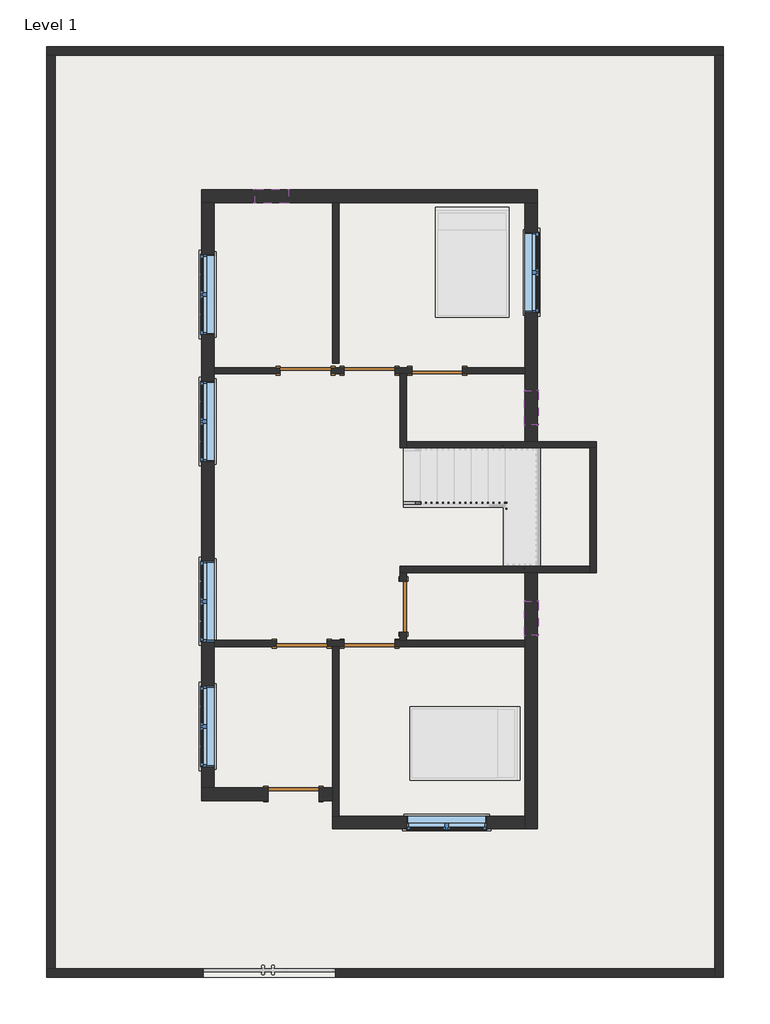
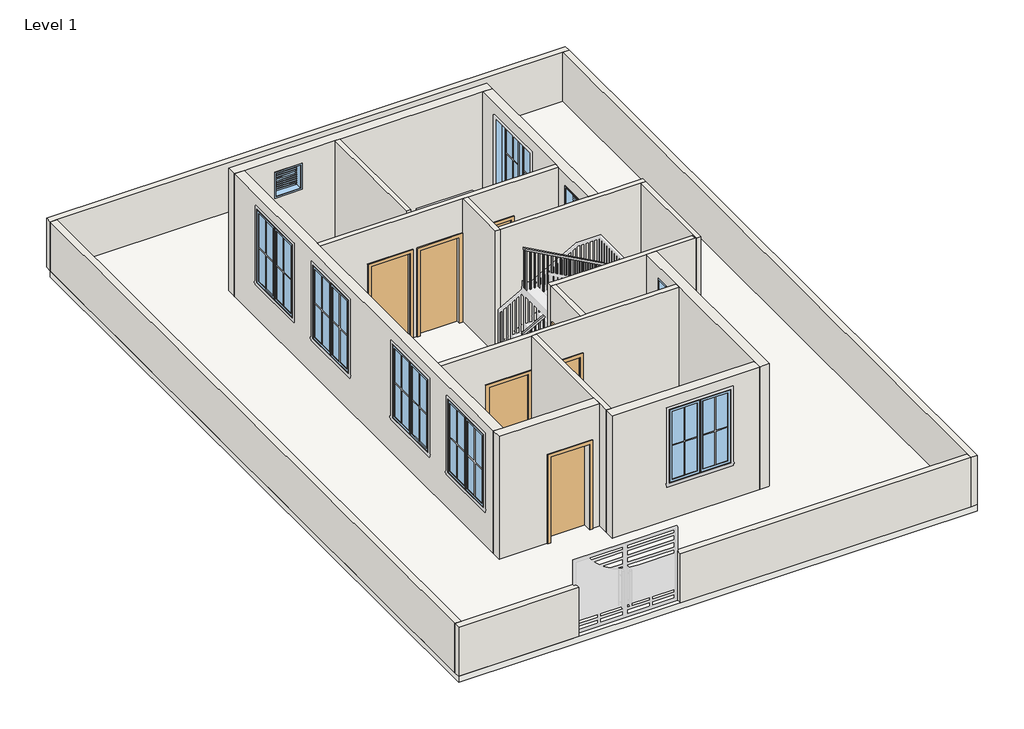
# One storey, part 1 of 2: 20 walls, 9 windows, 7 doors, 1 railing, 1 slab.
"""IFC4 building model written with IfcOpenShell, lengths in millimetres."""

from ifc_helpers import new_model, si_unit, frame, origin, origin_with_axes, place, context, project, spatial, polyline, outline, extrude, faceted_brep, transform, mapped, element, save
from components import door_e5f9f3c4, door_305aa2a5, door_0ca8825f, window_9ac97e1a, window_f2d8fef0

model = new_model("IFC4")

# Units and contexts
model_context = context("Model", 3, world=origin())
ifc_project = project(units=[si_unit("LENGTHUNIT", "METRE", prefix="MILLI")], contexts=[model_context])

# Site, building, storey
site = spatial("IfcSite", under=ifc_project)
building = spatial("IfcBuilding", under=site)
storey = spatial("IfcBuildingStorey", under=building, Name="Level 1", Elevation=0.0)

# Doors
placement = place(None, origin())
door_shape = door_e5f9f3c4(model_context)
element("IfcDoor", 1, ObjectType="Single-Flush : 36\" x 84\"", at=placement, inside=storey, context=model_context, shape_type="MappedRepresentation", body=[
    mapped(door_shape, transform((-2929.7888307, 2238.9017201, 0.0), x_axis=(1.0, 0.0, 0.0), y_axis=(0.0, 1.0, 0.0), z_axis=(0.0, 0.0, 1.0))),
])
element("IfcDoor", 2, ObjectType="Single-Flush : 36\" x 84\"", at=placement, inside=storey, context=model_context, shape_type="MappedRepresentation", body=[
    mapped(door_shape, transform((-558.0638307, 2238.9017201, 0.0), x_axis=(-1.0, 0.0, 0.0), y_axis=(0.0, -1.0, 0.0), z_axis=(0.0, 0.0, 1.0))),
])
element("IfcDoor", 3, ObjectType="Single-Flush : 36\" x 84\"", at=placement, inside=storey, context=model_context, shape_type="MappedRepresentation", body=[
    mapped(door_shape, transform((-1167.6638307, -2009.2482799, 0.0), x_axis=(0.0, -1.0, 0.0), y_axis=(1.0, 0.0, 0.0), z_axis=(0.0, 0.0, 1.0))),
])
element("IfcDoor", 4, ObjectType="Single-Flush : 36\" x 84\"", at=placement, inside=storey, context=model_context, shape_type="MappedRepresentation", body=[
    mapped(door_shape, transform((-1777.2638307, -2675.9982799, 0.0), x_axis=(-1.0, 0.0, 0.0), y_axis=(0.0, -1.0, 0.0), z_axis=(0.0, 0.0, 1.0))),
])
door_2_shape = door_305aa2a5(model_context)
element("IfcDoor", 5, ObjectType="Single-Flush : 36\" x 84\"", at=placement, inside=storey, context=model_context, shape_type="MappedRepresentation", body=[
    mapped(door_2_shape, transform((-1777.2638307, 2238.9017201, 0.0), x_axis=(-1.0, 0.0, 0.0), y_axis=(0.0, -1.0, 0.0), z_axis=(0.0, 0.0, 1.0))),
])
element("IfcDoor", 6, ObjectType="Single-Flush : 36\" x 84\"", at=placement, inside=storey, context=model_context, shape_type="MappedRepresentation", body=[
    mapped(door_2_shape, transform((-2996.4638307, -2675.9982799, 0.0), x_axis=(1.0, 0.0, 0.0), y_axis=(0.0, 1.0, 0.0), z_axis=(0.0, 0.0, 1.0))),
])
door_3_shape = door_0ca8825f(model_context)
element("IfcDoor", 7, ObjectType="Single-Flush : 36\" x 84\"", at=placement, inside=storey, context=model_context, shape_type="MappedRepresentation", body=[
    mapped(door_3_shape, transform((-3148.8638307, -5387.4482799, 0.0), x_axis=(1.0, 0.0, 0.0), y_axis=(0.0, 1.0, 0.0), z_axis=(0.0, 0.0, 1.0))),
])

# Railing
element("IfcRailing", 8, ObjectType="Handrail - Rectangular", at=placement, inside=storey, context=model_context, shape_type="SolidModel", body=[
    faceted_brep([(-1167.6638307, -116.9482799, 1083.7333333), (-1167.6638307, -116.9482799, 1025.6675836), (-1167.6638307, -167.7482799, 1025.6675836), (-1167.6638307, -167.7482799, 1083.7333333), (591.2861693, -116.9482799, 2057.5464821), (642.0861693, -116.9482799, 2027.6052998), (642.0861693, -167.7482799, 2027.6052998), (591.2861693, -167.7482799, 2057.5464821), (591.2861693, -116.9482799, 2099.7333333), (642.0861693, -116.9482799, 2048.9333333), (642.0861693, -167.7482799, 2048.9333333), (591.2861693, -167.7482799, 2099.7333333), (718.2861693, -116.9482799, 2099.7333333), (718.2861693, -116.9482799, 2048.9333333), (667.4861693, -167.7482799, 2048.9333333), (667.4861693, -167.7482799, 2099.7333333), (718.2861693, -218.5482799, 2099.7333333), (667.4861693, -218.5482799, 2099.7333333), (667.4861693, -269.3482799, 2048.9333333), (718.2861693, -269.3482799, 2048.9333333)], [[[0, 1, 2, 3]], [[1, 0, 4, 5]], [[2, 1, 5, 6]], [[3, 2, 6, 7]], [[0, 3, 7, 4]], [[5, 4, 8, 9]], [[6, 5, 9, 10]], [[7, 6, 10, 11]], [[4, 7, 11, 8]], [[9, 8, 12, 13]], [[10, 9, 13, 14]], [[11, 10, 14, 15]], [[8, 11, 15, 12]], [[16, 17, 18, 19]], [[13, 12, 16, 19]], [[14, 13, 19, 18]], [[15, 14, 18, 17]], [[12, 15, 17, 16]]]),
    faceted_brep([(718.2861693, -218.5482799, 2099.7333333), (718.2861693, -269.3482799, 2048.9333333), (667.4861693, -269.3482799, 2048.9333333), (667.4861693, -218.5482799, 2099.7333333), (718.2861693, -218.5482799, 2241.2310502), (667.4861693, -218.5482799, 2211.1403208), (667.4861693, -269.3482799, 2211.1403208), (718.2861693, -269.3482799, 2241.2310502)], [[[0, 1, 2, 3]], [[4, 5, 6, 7]], [[1, 0, 4, 7]], [[2, 1, 7, 6]], [[3, 2, 6, 5]], [[0, 3, 5, 4]]]),
    faceted_brep([(718.2861693, -269.3482799, 2241.2310502), (667.4861693, -269.3482799, 2211.1403208), (667.4861693, -218.5482799, 2211.1403208), (718.2861693, -218.5482799, 2241.2310502), (-1186.7138307, -269.3482799, 3285.0666667), (-1186.7138307, -218.5482799, 3285.0666667), (-1186.7138307, -218.5482799, 3227.1403208), (-1186.7138307, -269.3482799, 3227.1403208)], [[[0, 1, 2, 3]], [[4, 5, 6, 7]], [[1, 0, 4, 7]], [[2, 1, 7, 6]], [[3, 2, 6, 5]], [[0, 3, 5, 4]]]),
    extrude(outline(polyline([(3194.0855263, -1126.3888307), (3204.5238825, -1145.4388307), (2201.3333333, -1145.4388307), (2201.3333333, -1126.3888307), (3194.0855263, -1126.3888307)])), frame((0.0, -253.4732799, 0.0), z_axis=(0.0, 1.0, 0.0), x_axis=(0.0, 0.0, 1.0)), (0.0, 0.0, 1.0), 19.05),
    extrude(outline(polyline([(3138.4142934, -1024.7888307), (3148.8526496, -1043.8388307), (2201.3333333, -1043.8388307), (2201.3333333, -1024.7888307), (3138.4142934, -1024.7888307)])), frame((0.0, -253.4732799, 0.0), z_axis=(0.0, 1.0, 0.0), x_axis=(0.0, 0.0, 1.0)), (0.0, 0.0, 1.0), 19.05),
    extrude(outline(polyline([(3082.7430606, -923.1888307), (3093.1814167, -942.2388307), (2201.3333333, -942.2388307), (2201.3333333, -923.1888307), (3082.7430606, -923.1888307)])), frame((0.0, -253.4732799, 0.0), z_axis=(0.0, 1.0, 0.0), x_axis=(0.0, 0.0, 1.0)), (0.0, 0.0, 1.0), 19.05),
    extrude(outline(polyline([(3027.0718277, -821.5888307), (3037.5101838, -840.6388307), (2032.0, -840.6388307), (2032.0, -821.5888307), (3027.0718277, -821.5888307)])), frame((0.0, -253.4732799, 0.0), z_axis=(0.0, 1.0, 0.0), x_axis=(0.0, 0.0, 1.0)), (0.0, 0.0, 1.0), 19.05),
    extrude(outline(polyline([(2971.4005948, -719.9888307), (2981.838951, -739.0388307), (2032.0, -739.0388307), (2032.0, -719.9888307), (2971.4005948, -719.9888307)])), frame((0.0, -253.4732799, 0.0), z_axis=(0.0, 1.0, 0.0), x_axis=(0.0, 0.0, 1.0)), (0.0, 0.0, 1.0), 19.05),
    extrude(outline(polyline([(2915.7293619, -618.3888307), (2926.1677181, -637.4388307), (2032.0, -637.4388307), (2032.0, -618.3888307), (2915.7293619, -618.3888307)])), frame((0.0, -253.4732799, 0.0), z_axis=(0.0, 1.0, 0.0), x_axis=(0.0, 0.0, 1.0)), (0.0, 0.0, 1.0), 19.05),
    extrude(outline(polyline([(2860.058129, -516.7888307), (2870.4964852, -535.8388307), (1862.6666667, -535.8388307), (1862.6666667, -516.7888307), (2860.058129, -516.7888307)])), frame((0.0, -253.4732799, 0.0), z_axis=(0.0, 1.0, 0.0), x_axis=(0.0, 0.0, 1.0)), (0.0, 0.0, 1.0), 19.05),
    extrude(outline(polyline([(2804.3868962, -415.1888307), (2814.8252523, -434.2388307), (1862.6666667, -434.2388307), (1862.6666667, -415.1888307), (2804.3868962, -415.1888307)])), frame((0.0, -253.4732799, 0.0), z_axis=(0.0, 1.0, 0.0), x_axis=(0.0, 0.0, 1.0)), (0.0, 0.0, 1.0), 19.05),
    extrude(outline(polyline([(2748.7156633, -313.5888307), (2759.1540195, -332.6388307), (1862.6666667, -332.6388307), (1862.6666667, -313.5888307), (2748.7156633, -313.5888307)])), frame((0.0, -253.4732799, 0.0), z_axis=(0.0, 1.0, 0.0), x_axis=(0.0, 0.0, 1.0)), (0.0, 0.0, 1.0), 19.05),
    extrude(outline(polyline([(2693.0444304, -211.9888307), (2703.4827866, -231.0388307), (1693.3333333, -231.0388307), (1693.3333333, -211.9888307), (2693.0444304, -211.9888307)])), frame((0.0, -253.4732799, 0.0), z_axis=(0.0, 1.0, 0.0), x_axis=(0.0, 0.0, 1.0)), (0.0, 0.0, 1.0), 19.05),
    extrude(outline(polyline([(2637.3731975, -110.3888307), (2647.8115537, -129.4388307), (1693.3333333, -129.4388307), (1693.3333333, -110.3888307), (2637.3731975, -110.3888307)])), frame((0.0, -253.4732799, 0.0), z_axis=(0.0, 1.0, 0.0), x_axis=(0.0, 0.0, 1.0)), (0.0, 0.0, 1.0), 19.05),
    extrude(outline(polyline([(2581.7019647, -8.7888307), (2592.1403208, -27.8388307), (1693.3333333, -27.8388307), (1693.3333333, -8.7888307), (2581.7019647, -8.7888307)])), frame((0.0, -253.4732799, 0.0), z_axis=(0.0, 1.0, 0.0), x_axis=(0.0, 0.0, 1.0)), (0.0, 0.0, 1.0), 19.05),
    extrude(outline(polyline([(2526.0307318, 92.8111693), (2536.4690879, 73.7611693), (1524.0, 73.7611693), (1524.0, 92.8111693), (2526.0307318, 92.8111693)])), frame((0.0, -253.4732799, 0.0), z_axis=(0.0, 1.0, 0.0), x_axis=(0.0, 0.0, 1.0)), (0.0, 0.0, 1.0), 19.05),
    extrude(outline(polyline([(2470.3594989, 194.4111693), (2480.7978551, 175.3611693), (1524.0, 175.3611693), (1524.0, 194.4111693), (2470.3594989, 194.4111693)])), frame((0.0, -253.4732799, 0.0), z_axis=(0.0, 1.0, 0.0), x_axis=(0.0, 0.0, 1.0)), (0.0, 0.0, 1.0), 19.05),
    extrude(outline(polyline([(2414.688266, 296.0111693), (2425.1266222, 276.9611693), (1524.0, 276.9611693), (1524.0, 296.0111693), (2414.688266, 296.0111693)])), frame((0.0, -253.4732799, 0.0), z_axis=(0.0, 1.0, 0.0), x_axis=(0.0, 0.0, 1.0)), (0.0, 0.0, 1.0), 19.05),
    extrude(outline(polyline([(2359.0170332, 397.6111693), (2369.4553893, 378.5611693), (1354.6666667, 378.5611693), (1354.6666667, 397.6111693), (2359.0170332, 397.6111693)])), frame((0.0, -253.4732799, 0.0), z_axis=(0.0, 1.0, 0.0), x_axis=(0.0, 0.0, 1.0)), (0.0, 0.0, 1.0), 19.05),
    extrude(outline(polyline([(2303.3458003, 499.2111693), (2313.7841564, 480.1611693), (1354.6666667, 480.1611693), (1354.6666667, 499.2111693), (2303.3458003, 499.2111693)])), frame((0.0, -253.4732799, 0.0), z_axis=(0.0, 1.0, 0.0), x_axis=(0.0, 0.0, 1.0)), (0.0, 0.0, 1.0), 19.05),
    extrude(outline(polyline([(2247.6745674, 600.8111693), (2258.1129236, 581.7611693), (1354.6666667, 581.7611693), (1354.6666667, 600.8111693), (2247.6745674, 600.8111693)])), frame((0.0, -253.4732799, 0.0), z_axis=(0.0, 1.0, 0.0), x_axis=(0.0, 0.0, 1.0)), (0.0, 0.0, 1.0), 19.05),
    extrude(outline(polyline([(651.6111693, -151.8732799), (651.6111693, -132.8232799), (670.6611693, -132.8232799), (670.6611693, -151.8732799), (651.6111693, -151.8732799)])), frame((0.0, 0.0, 1016.0), z_axis=(0.0, 0.0, 1.0), x_axis=(1.0, 0.0, 0.0)), (0.0, 0.0, 1.0), 1032.9333333),
    extrude(outline(polyline([(1987.1762341, 569.0611693), (1976.6295213, 550.0111693), (1016.0, 550.0111693), (1016.0, 569.0611693), (1987.1762341, 569.0611693)])), frame((0.0, -151.8732799, 0.0), z_axis=(0.0, 1.0, 0.0), x_axis=(0.0, 0.0, 1.0)), (0.0, 0.0, 1.0), 19.05),
    extrude(outline(polyline([(1930.9270991, 467.4611693), (1920.3803863, 448.4111693), (1016.0, 448.4111693), (1016.0, 467.4611693), (1930.9270991, 467.4611693)])), frame((0.0, -151.8732799, 0.0), z_axis=(0.0, 1.0, 0.0), x_axis=(0.0, 0.0, 1.0)), (0.0, 0.0, 1.0), 19.05),
    extrude(outline(polyline([(1874.6779642, 365.8611693), (1864.1312514, 346.8111693), (846.6666667, 346.8111693), (846.6666667, 365.8611693), (1874.6779642, 365.8611693)])), frame((0.0, -151.8732799, 0.0), z_axis=(0.0, 1.0, 0.0), x_axis=(0.0, 0.0, 1.0)), (0.0, 0.0, 1.0), 19.05),
    extrude(outline(polyline([(1818.4288292, 264.2611693), (1807.8821164, 245.2111693), (846.6666667, 245.2111693), (846.6666667, 264.2611693), (1818.4288292, 264.2611693)])), frame((0.0, -151.8732799, 0.0), z_axis=(0.0, 1.0, 0.0), x_axis=(0.0, 0.0, 1.0)), (0.0, 0.0, 1.0), 19.05),
    extrude(outline(polyline([(1762.1796943, 162.6611693), (1751.6329815, 143.6111693), (846.6666667, 143.6111693), (846.6666667, 162.6611693), (1762.1796943, 162.6611693)])), frame((0.0, -151.8732799, 0.0), z_axis=(0.0, 1.0, 0.0), x_axis=(0.0, 0.0, 1.0)), (0.0, 0.0, 1.0), 19.05),
    extrude(outline(polyline([(1705.9305593, 61.0611693), (1695.3838465, 42.0111693), (677.3333333, 42.0111693), (677.3333333, 61.0611693), (1705.9305593, 61.0611693)])), frame((0.0, -151.8732799, 0.0), z_axis=(0.0, 1.0, 0.0), x_axis=(0.0, 0.0, 1.0)), (0.0, 0.0, 1.0), 19.05),
    extrude(outline(polyline([(1649.6814244, -40.5388307), (1639.1347116, -59.5888307), (677.3333333, -59.5888307), (677.3333333, -40.5388307), (1649.6814244, -40.5388307)])), frame((0.0, -151.8732799, 0.0), z_axis=(0.0, 1.0, 0.0), x_axis=(0.0, 0.0, 1.0)), (0.0, 0.0, 1.0), 19.05),
    extrude(outline(polyline([(1593.4322895, -142.1388307), (1582.8855766, -161.1888307), (677.3333333, -161.1888307), (677.3333333, -142.1388307), (1593.4322895, -142.1388307)])), frame((0.0, -151.8732799, 0.0), z_axis=(0.0, 1.0, 0.0), x_axis=(0.0, 0.0, 1.0)), (0.0, 0.0, 1.0), 19.05),
    extrude(outline(polyline([(1537.1831545, -243.7388307), (1526.6364417, -262.7888307), (508.0, -262.7888307), (508.0, -243.7388307), (1537.1831545, -243.7388307)])), frame((0.0, -151.8732799, 0.0), z_axis=(0.0, 1.0, 0.0), x_axis=(0.0, 0.0, 1.0)), (0.0, 0.0, 1.0), 19.05),
    extrude(outline(polyline([(1480.9340196, -345.3388307), (1470.3873068, -364.3888307), (508.0, -364.3888307), (508.0, -345.3388307), (1480.9340196, -345.3388307)])), frame((0.0, -151.8732799, 0.0), z_axis=(0.0, 1.0, 0.0), x_axis=(0.0, 0.0, 1.0)), (0.0, 0.0, 1.0), 19.05),
    extrude(outline(polyline([(1424.6848846, -446.9388307), (1414.1381718, -465.9888307), (508.0, -465.9888307), (508.0, -446.9388307), (1424.6848846, -446.9388307)])), frame((0.0, -151.8732799, 0.0), z_axis=(0.0, 1.0, 0.0), x_axis=(0.0, 0.0, 1.0)), (0.0, 0.0, 1.0), 19.05),
    extrude(outline(polyline([(1368.4357497, -548.5388307), (1357.8890369, -567.5888307), (338.6666667, -567.5888307), (338.6666667, -548.5388307), (1368.4357497, -548.5388307)])), frame((0.0, -151.8732799, 0.0), z_axis=(0.0, 1.0, 0.0), x_axis=(0.0, 0.0, 1.0)), (0.0, 0.0, 1.0), 19.05),
    extrude(outline(polyline([(1312.1866147, -650.1388307), (1301.6399019, -669.1888307), (338.6666667, -669.1888307), (338.6666667, -650.1388307), (1312.1866147, -650.1388307)])), frame((0.0, -151.8732799, 0.0), z_axis=(0.0, 1.0, 0.0), x_axis=(0.0, 0.0, 1.0)), (0.0, 0.0, 1.0), 19.05),
    extrude(outline(polyline([(1255.9374798, -751.7388307), (1245.390767, -770.7888307), (338.6666667, -770.7888307), (338.6666667, -751.7388307), (1255.9374798, -751.7388307)])), frame((0.0, -151.8732799, 0.0), z_axis=(0.0, 1.0, 0.0), x_axis=(0.0, 0.0, 1.0)), (0.0, 0.0, 1.0), 19.05),
    extrude(outline(polyline([(1199.6883448, -853.3388307), (1189.141632, -872.3888307), (169.3333333, -872.3888307), (169.3333333, -853.3388307), (1199.6883448, -853.3388307)])), frame((0.0, -151.8732799, 0.0), z_axis=(0.0, 1.0, 0.0), x_axis=(0.0, 0.0, 1.0)), (0.0, 0.0, 1.0), 19.05),
    extrude(outline(polyline([(1143.4392099, -954.9388307), (1132.8924971, -973.9888307), (169.3333333, -973.9888307), (169.3333333, -954.9388307), (1143.4392099, -954.9388307)])), frame((0.0, -151.8732799, 0.0), z_axis=(0.0, 1.0, 0.0), x_axis=(0.0, 0.0, 1.0)), (0.0, 0.0, 1.0), 19.05),
    extrude(outline(polyline([(1087.1900749, -1056.5388307), (1076.6433621, -1075.5888307), (169.3333333, -1075.5888307), (169.3333333, -1056.5388307), (1087.1900749, -1056.5388307)])), frame((0.0, -151.8732799, 0.0), z_axis=(0.0, 1.0, 0.0), x_axis=(0.0, 0.0, 1.0)), (0.0, 0.0, 1.0), 19.05),
    extrude(outline(polyline([(683.3611693, -234.4232799), (702.4111693, -234.4232799), (702.4111693, -253.4732799), (683.3611693, -253.4732799), (683.3611693, -234.4232799)])), frame((0.0, 0.0, 1185.3333333), z_axis=(0.0, 0.0, 1.0), x_axis=(1.0, 0.0, 0.0)), (0.0, 0.0, 1.0), 863.6),
    extrude(outline(polyline([(683.3611693, -151.8732799), (683.3611693, -132.8232799), (702.4111693, -132.8232799), (702.4111693, -151.8732799), (683.3611693, -151.8732799)])), frame((0.0, 0.0, 1185.3333333), z_axis=(0.0, 0.0, 1.0), x_axis=(1.0, 0.0, 0.0)), (0.0, 0.0, 1.0), 863.6),
    extrude(outline(polyline([(3216.7019647, -1167.6638307), (3227.1403208, -1186.7138307), (2201.3333333, -1186.7138307), (2201.3333333, -1167.6638307), (3216.7019647, -1167.6638307)])), frame((0.0, -253.4732799, 0.0), z_axis=(0.0, 1.0, 0.0), x_axis=(0.0, 0.0, 1.0)), (0.0, 0.0, 1.0), 19.05),
    extrude(outline(polyline([(1036.2142964, -1148.6138307), (1025.6675836, -1167.6638307), (169.3333333, -1167.6638307), (169.3333333, -1148.6138307), (1036.2142964, -1148.6138307)])), frame((0.0, -151.8732799, 0.0), z_axis=(0.0, 1.0, 0.0), x_axis=(0.0, 0.0, 1.0)), (0.0, 0.0, 1.0), 19.05),
])

# Slab
element("IfcSlab", 9, ObjectType="FLOOR 6\"", at=placement, inside=storey, context=model_context, shape_type="SweptSolid", body=[
    extrude(outline(polyline([(4593.8462821, 7924.3928796), (4593.8462821, -8687.2071204), (-7598.1537179, -8687.2071204), (-7598.1537179, 7924.3928796), (4593.8462821, 7924.3928796)])), frame((0.0, 0.0, -152.4), z_axis=(0.0, 0.0, 1.0), x_axis=(1.0, 0.0, 0.0)), (0.0, 0.0, 1.0), 152.4),
])

# Walls
element("IfcWall", 10, ObjectType="CMD 6\"", at=placement, inside=storey, context=model_context, shape_type="Brep", body=[
    faceted_brep([(-7598.1537179, 7924.3928796, 0.0), (-7445.7537179, 7924.3928796, 0.0), (4441.4462821, 7924.3928796, 0.0), (4593.8462821, 7924.3928796, 0.0), (4593.8462821, 7924.3928796, 1219.2), (4441.4462821, 7924.3928796, 1219.2), (-7445.7537179, 7924.3928796, 1219.2), (-7598.1537179, 7924.3928796, 1219.2), (-7598.1537179, 8076.7928796, 0.0), (-7598.1537179, 8076.7928796, 1219.2), (4593.8462821, 8076.7928796, 1219.2), (4593.8462821, 8076.7928796, 0.0)], [[[0, 1, 2, 3, 4, 5, 6, 7]], [[8, 9, 10, 11]], [[3, 2, 1, 0, 8, 11]], [[7, 6, 5, 4, 10, 9]], [[4, 3, 11, 10]], [[0, 7, 9, 8]]]),
])
element("IfcWall", 11, ObjectType="CMD 6\"", at=placement, inside=storey, context=model_context, shape_type="Brep", body=[
    faceted_brep([(4441.4462821, 7924.3928796, 0.0), (4441.4462821, -8534.8071204, 0.0), (4441.4462821, -8687.2071204, 0.0), (4441.4462821, -8687.2071204, 1219.2), (4441.4462821, -8534.8071204, 1219.2), (4441.4462821, 7924.3928796, 1219.2), (4593.8462821, 7924.3928796, 0.0), (4593.8462821, 7924.3928796, 1219.2), (4593.8462821, -8687.2071204, 1219.2), (4593.8462821, -8687.2071204, 0.0)], [[[0, 1, 2, 3, 4, 5]], [[6, 7, 8, 9]], [[2, 1, 0, 6, 9]], [[5, 4, 3, 8, 7]], [[0, 5, 7, 6]], [[3, 2, 9, 8]]]),
])
element("IfcWall", 12, ObjectType="CMD 6\"", at=placement, inside=storey, context=model_context, shape_type="SweptSolid", body=[
    extrude(outline(polyline([(-2386.8638307, -8534.8071204), (4441.4462821, -8534.8071204), (4441.4462821, -8687.2071204), (-2386.8638307, -8687.2071204), (-2386.8638307, -8534.8071204)])), origin_with_axes(), (0.0, 0.0, 1.0), 1219.2),
])
element("IfcWall", 13, ObjectType="CMD 6\"", at=placement, inside=storey, context=model_context, shape_type="SweptSolid", body=[
    extrude(outline(polyline([(-7445.7537179, 7924.3928796), (-7445.7537179, -8534.8071204), (-7598.1537179, -8534.8071204), (-7598.1537179, 7924.3928796), (-7445.7537179, 7924.3928796)])), origin_with_axes(), (0.0, 0.0, 1.0), 1219.2),
])
element("IfcWall", 14, ObjectType="CMD 6\"", at=placement, inside=storey, context=model_context, shape_type="Brep", body=[
    faceted_brep([(-4774.4638307, -8534.8071204, 0.0), (-7445.7537179, -8534.8071204, 0.0), (-7598.1537179, -8534.8071204, 0.0), (-7598.1537179, -8534.8071204, 1219.2), (-7445.7537179, -8534.8071204, 1219.2), (-4774.4638307, -8534.8071204, 1219.2), (-4774.4638307, -8687.2071204, 0.0), (-4774.4638307, -8687.2071204, 1219.2), (-7598.1537179, -8687.2071204, 1219.2), (-7598.1537179, -8687.2071204, 0.0)], [[[0, 1, 2, 3, 4, 5]], [[6, 7, 8, 9]], [[2, 1, 0, 6, 9]], [[5, 4, 3, 8, 7]], [[0, 5, 7, 6]], [[3, 2, 9, 8]]]),
])
element("IfcWall", 15, ObjectType="WALL 4.5\"", at=placement, inside=storey, context=model_context, shape_type="SweptSolid", body=[
    extrude(outline(polyline([(-2444.0138307, 2372.2517201), (-2444.0138307, 5267.8517201), (-2329.7138307, 5267.8517201), (-2329.7138307, 2372.2517201), (-2444.0138307, 2372.2517201)])), origin_with_axes(), (0.0, 0.0, 1.0), 3048.0),
])
element("IfcWall", 16, ObjectType="WALL 4.5\"", at=placement, inside=storey, context=model_context, shape_type="Brep", body=[
    faceted_brep([(-1320.0638307, 2181.7517201, 0.0), (-1224.8138307, 2181.7517201, 0.0), (-1110.5138307, 2181.7517201, 0.0), (-1015.2638307, 2181.7517201, 0.0), (-1015.2638307, 2181.7517201, 2133.6), (-100.8638307, 2181.7517201, 2133.6), (-100.8638307, 2181.7517201, 0.0), (1023.0861693, 2181.7517201, 0.0), (1023.0861693, 2181.7517201, 3048.0), (-1110.5138307, 2181.7517201, 3048.0), (-1224.8138307, 2181.7517201, 3048.0), (-4577.6138307, 2181.7517201, 3048.0), (-4577.6138307, 2181.7517201, 0.0), (-3386.9888307, 2181.7517201, 0.0), (-3386.9888307, 2181.7517201, 2133.6), (-2472.5888307, 2181.7517201, 2133.6), (-2472.5888307, 2181.7517201, 0.0), (-2234.4638307, 2181.7517201, 0.0), (-2234.4638307, 2181.7517201, 2133.6), (-1320.0638307, 2181.7517201, 2133.6), (-1015.2638307, 2296.0517201, 2133.6), (-1015.2638307, 2296.0517201, 0.0), (-1320.0638307, 2296.0517201, 0.0), (-1320.0638307, 2296.0517201, 2133.6), (-2234.4638307, 2296.0517201, 2133.6), (-2234.4638307, 2296.0517201, 0.0), (-2472.5888307, 2296.0517201, 0.0), (-2472.5888307, 2296.0517201, 2133.6), (-3386.9888307, 2296.0517201, 2133.6), (-3386.9888307, 2296.0517201, 0.0), (-4577.6138307, 2296.0517201, 0.0), (-4577.6138307, 2296.0517201, 3048.0), (1023.0861693, 2296.0517201, 3048.0), (1023.0861693, 2296.0517201, 0.0), (-100.8638307, 2296.0517201, 0.0), (-100.8638307, 2296.0517201, 2133.6)], [[[0, 1, 2, 3, 4, 5, 6, 7, 8, 9, 10, 11, 12, 13, 14, 15, 16, 17, 18, 19]], [[20, 21, 22, 23, 24, 25, 26, 27, 28, 29, 30, 31, 32, 33, 34, 35]], [[13, 12, 30, 29]], [[26, 25, 17, 16]], [[34, 33, 7, 6]], [[22, 21, 3, 2, 1, 0]], [[8, 7, 33, 32]], [[12, 11, 31, 30]], [[27, 26, 16, 15]], [[28, 27, 15, 14]], [[29, 28, 14, 13]], [[18, 17, 25, 24]], [[19, 18, 24, 23]], [[0, 19, 23, 22]], [[4, 3, 21, 20]], [[5, 4, 20, 35]], [[6, 5, 35, 34]], [[11, 10, 9, 8, 32, 31]]]),
])
element("IfcWall", 17, ObjectType="WALL 4.5\"", at=placement, inside=storey, context=model_context, shape_type="Brep", body=[
    faceted_brep([(-1224.8138307, 2181.7517201, 0.0), (-1224.8138307, 848.2517201, 0.0), (-1224.8138307, 848.2517201, 3048.0), (-1224.8138307, 2181.7517201, 3048.0), (-1110.5138307, 2181.7517201, 0.0), (-1110.5138307, 2181.7517201, 3048.0), (-1110.5138307, 962.5517201, 3048.0), (-1110.5138307, 848.2517201, 3048.0), (-1110.5138307, 848.2517201, 0.0), (-1110.5138307, 962.5517201, 0.0)], [[[0, 1, 2, 3]], [[4, 5, 6, 7, 8, 9]], [[1, 0, 4, 9, 8]], [[0, 3, 5, 4]], [[2, 1, 8, 7]], [[3, 2, 7, 6, 5]]]),
])
element("IfcWall", 18, ObjectType="WALL 4.5\"", at=placement, inside=storey, context=model_context, shape_type="Brep", body=[
    faceted_brep([(-1110.5138307, 848.2517201, 0.0), (2191.4861693, 848.2517201, 0.0), (2305.7861693, 848.2517201, 0.0), (2305.7861693, 848.2517201, 3048.0), (2191.4861693, 848.2517201, 3048.0), (-1110.5138307, 848.2517201, 3048.0), (-1110.5138307, 962.5517201, 0.0), (-1110.5138307, 962.5517201, 3048.0), (1023.0861693, 962.5517201, 3048.0), (1251.6861693, 962.5517201, 3048.0), (2305.7861693, 962.5517201, 3048.0), (2305.7861693, 962.5517201, 0.0), (1251.6861693, 962.5517201, 0.0), (1023.0861693, 962.5517201, 0.0)], [[[0, 1, 2, 3, 4, 5]], [[6, 7, 8, 9, 10, 11, 12, 13]], [[2, 1, 0, 6, 13, 12, 11]], [[5, 4, 3, 10, 9, 8, 7]], [[0, 5, 7, 6]], [[3, 2, 11, 10]]]),
])
element("IfcWall", 19, ObjectType="WALL 4.5\"", at=placement, inside=storey, context=model_context, shape_type="Brep", body=[
    faceted_brep([(2191.4861693, 848.2517201, 0.0), (2191.4861693, -1285.3482799, 0.0), (2191.4861693, -1399.6482799, 0.0), (2191.4861693, -1399.6482799, 3048.0), (2191.4861693, -1285.3482799, 3048.0), (2191.4861693, 848.2517201, 3048.0), (2305.7861693, 848.2517201, 0.0), (2305.7861693, 848.2517201, 3048.0), (2305.7861693, -1399.6482799, 3048.0), (2305.7861693, -1399.6482799, 0.0)], [[[0, 1, 2, 3, 4, 5]], [[6, 7, 8, 9]], [[2, 1, 0, 6, 9]], [[5, 4, 3, 8, 7]], [[0, 5, 7, 6]], [[3, 2, 9, 8]]]),
])
element("IfcWall", 20, ObjectType="WALL 4.5\"", at=placement, inside=storey, context=model_context, shape_type="Brep", body=[
    faceted_brep([(2191.4861693, -1285.3482799, 0.0), (-1224.8138307, -1285.3482799, 0.0), (-1224.8138307, -1285.3482799, 3048.0), (-881.9138307, -1285.3482799, 3048.0), (1251.6861693, -1285.3482799, 3048.0), (2166.0861693, -1285.3482799, 3048.0), (2191.4861693, -1285.3482799, 3048.0), (2191.4861693, -1399.6482799, 0.0), (2191.4861693, -1399.6482799, 3048.0), (2166.0861693, -1399.6482799, 3048.0), (1251.6861693, -1399.6482799, 3048.0), (1023.0861693, -1399.6482799, 3048.0), (-1110.5138307, -1399.6482799, 3048.0), (-1224.8138307, -1399.6482799, 3048.0), (-1224.8138307, -1399.6482799, 0.0), (-1110.5138307, -1399.6482799, 0.0), (1023.0861693, -1399.6482799, 0.0), (1251.6861693, -1399.6482799, 0.0)], [[[0, 1, 2, 3, 4, 5, 6]], [[7, 8, 9, 10, 11, 12, 13, 14, 15, 16, 17]], [[1, 0, 7, 17, 16, 15, 14]], [[0, 6, 8, 7]], [[2, 1, 14, 13]], [[6, 5, 9, 8]], [[5, 4, 3, 2, 13, 12, 11, 10, 9]]]),
])
element("IfcWall", 21, ObjectType="WALL 4.5\"", at=placement, inside=storey, context=model_context, shape_type="SweptSolid", body=[
    extrude(outline(polyline([(-2466.4482799, 2133.6), (-2466.4482799, 0.0), (-2618.8482799, 0.0), (-2618.8482799, 3048.0), (-1399.6482799, 3048.0), (-1399.6482799, 0.0), (-1552.0482799, 0.0), (-1552.0482799, 2133.6), (-2466.4482799, 2133.6)])), frame((-1224.8138307, 0.0, 0.0), z_axis=(1.0, 0.0, 0.0), x_axis=(0.0, 1.0, 0.0)), (0.0, 0.0, 1.0), 114.3),
])
element("IfcWall", 22, ObjectType="WALL 4.5\"", at=placement, inside=storey, context=model_context, shape_type="Brep", body=[
    faceted_brep([(-2234.4638307, -2618.8482799, 0.0), (-2539.2638307, -2618.8482799, 0.0), (-2539.2638307, -2618.8482799, 2133.6), (-3453.6638307, -2618.8482799, 2133.6), (-3453.6638307, -2618.8482799, 0.0), (-4577.6138307, -2618.8482799, 0.0), (-4577.6138307, -2618.8482799, 3048.0), (-1224.8138307, -2618.8482799, 3048.0), (-1110.5138307, -2618.8482799, 3048.0), (1023.0861693, -2618.8482799, 3048.0), (1023.0861693, -2618.8482799, 0.0), (-1110.5138307, -2618.8482799, 0.0), (-1224.8138307, -2618.8482799, 0.0), (-1320.0638307, -2618.8482799, 0.0), (-1320.0638307, -2618.8482799, 2133.6), (-2234.4638307, -2618.8482799, 2133.6), (-2539.2638307, -2733.1482799, 2133.6), (-2539.2638307, -2733.1482799, 0.0), (-2444.0138307, -2733.1482799, 0.0), (-2329.7138307, -2733.1482799, 0.0), (-2234.4638307, -2733.1482799, 0.0), (-2234.4638307, -2733.1482799, 2133.6), (-1320.0638307, -2733.1482799, 2133.6), (-1320.0638307, -2733.1482799, 0.0), (1023.0861693, -2733.1482799, 0.0), (1023.0861693, -2733.1482799, 3048.0), (-2329.7138307, -2733.1482799, 3048.0), (-2444.0138307, -2733.1482799, 3048.0), (-4577.6138307, -2733.1482799, 3048.0), (-4577.6138307, -2733.1482799, 0.0), (-3453.6638307, -2733.1482799, 0.0), (-3453.6638307, -2733.1482799, 2133.6)], [[[0, 1, 2, 3, 4, 5, 6, 7, 8, 9, 10, 11, 12, 13, 14, 15]], [[16, 17, 18, 19, 20, 21, 22, 23, 24, 25, 26, 27, 28, 29, 30, 31]], [[13, 12, 11, 10, 24, 23]], [[30, 29, 5, 4]], [[20, 19, 18, 17, 1, 0]], [[10, 9, 25, 24]], [[6, 5, 29, 28]], [[21, 20, 0, 15]], [[22, 21, 15, 14]], [[23, 22, 14, 13]], [[2, 1, 17, 16]], [[3, 2, 16, 31]], [[4, 3, 31, 30]], [[9, 8, 7, 6, 28, 27, 26, 25]]]),
])
element("IfcWall", 23, ObjectType="WALL 4.5\"", at=placement, inside=storey, context=model_context, shape_type="Brep", body=[
    faceted_brep([(-2329.7138307, -5781.1482799, 0.0), (-2329.7138307, -2733.1482799, 0.0), (-2329.7138307, -2733.1482799, 3048.0), (-2329.7138307, -5781.1482799, 3048.0), (-2444.0138307, -5781.1482799, 0.0), (-2444.0138307, -5781.1482799, 3048.0), (-2444.0138307, -5501.7482799, 3048.0), (-2444.0138307, -5273.1482799, 3048.0), (-2444.0138307, -2733.1482799, 3048.0), (-2444.0138307, -2733.1482799, 0.0), (-2444.0138307, -5273.1482799, 0.0), (-2444.0138307, -5501.7482799, 0.0)], [[[0, 1, 2, 3]], [[4, 5, 6, 7, 8, 9, 10, 11]], [[1, 0, 4, 11, 10, 9]], [[0, 3, 5, 4]], [[2, 1, 9, 8]], [[3, 2, 8, 7, 6, 5]]]),
])
element("IfcWall", 24, ObjectType="WALL 9\"", at=placement, inside=storey, context=model_context, shape_type="Brep", body=[
    faceted_brep([(-4806.2138307, 5267.8517201, 0.0), (-4577.6138307, 5267.8517201, 0.0), (-2444.0138307, 5267.8517201, 0.0), (-2329.7138307, 5267.8517201, 0.0), (1023.0861693, 5267.8517201, 0.0), (1251.6861693, 5267.8517201, 0.0), (1251.6861693, 5267.8517201, 3048.0), (1023.0861693, 5267.8517201, 3048.0), (-2329.7138307, 5267.8517201, 3048.0), (-2444.0138307, 5267.8517201, 3048.0), (-4577.6138307, 5267.8517201, 3048.0), (-4806.2138307, 5267.8517201, 3048.0), (-3844.1888307, 5267.8517201, 2743.2), (-3234.5888307, 5267.8517201, 2743.2), (-3234.5888307, 5267.8517201, 2133.6), (-3844.1888307, 5267.8517201, 2133.6), (-4806.2138307, 5496.4517201, 0.0), (-4806.2138307, 5496.4517201, 3048.0), (1251.6861693, 5496.4517201, 3048.0), (1251.6861693, 5496.4517201, 0.0), (-3844.1888307, 5496.4517201, 2743.2), (-3844.1888307, 5496.4517201, 2133.6), (-3234.5888307, 5496.4517201, 2133.6), (-3234.5888307, 5496.4517201, 2743.2)], [[[0, 1, 2, 3, 4, 5, 6, 7, 8, 9, 10, 11], [12, 13, 14, 15]], [[16, 17, 18, 19], [20, 21, 22, 23]], [[5, 4, 3, 2, 1, 0, 16, 19]], [[6, 5, 19, 18]], [[0, 11, 17, 16]], [[21, 20, 12, 15]], [[22, 21, 15, 14]], [[23, 22, 14, 13]], [[20, 23, 13, 12]], [[11, 10, 9, 8, 7, 6, 18, 17]]]),
])
element("IfcWall", 25, ObjectType="WALL 9\"", at=placement, inside=storey, context=model_context, shape_type="Brep", body=[
    faceted_brep([(1023.0861693, 5267.8517201, 0.0), (1023.0861693, 2296.0517201, 0.0), (1023.0861693, 2181.7517201, 0.0), (1023.0861693, 962.5517201, 0.0), (1023.0861693, 962.5517201, 3048.0), (1023.0861693, 2181.7517201, 3048.0), (1023.0861693, 2296.0517201, 3048.0), (1023.0861693, 5267.8517201, 3048.0), (1023.0861693, 3286.6517201, 2743.2), (1023.0861693, 3286.6517201, 914.4), (1023.0861693, 4734.4517201, 914.4), (1023.0861693, 4734.4517201, 2743.2), (1023.0861693, 1876.9517201, 2743.2), (1023.0861693, 1267.3517201, 2743.2), (1023.0861693, 1267.3517201, 2133.6), (1023.0861693, 1876.9517201, 2133.6), (1251.6861693, 5267.8517201, 0.0), (1251.6861693, 5267.8517201, 3048.0), (1251.6861693, 962.5517201, 3048.0), (1251.6861693, 962.5517201, 0.0), (1251.6861693, 3286.6517201, 2743.2), (1251.6861693, 4734.4517201, 2743.2), (1251.6861693, 4734.4517201, 914.4), (1251.6861693, 3286.6517201, 914.4), (1251.6861693, 1876.9517201, 2743.2), (1251.6861693, 1876.9517201, 2133.6), (1251.6861693, 1267.3517201, 2133.6), (1251.6861693, 1267.3517201, 2743.2)], [[[0, 1, 2, 3, 4, 5, 6, 7], [8, 9, 10, 11], [12, 13, 14, 15]], [[16, 17, 18, 19], [20, 21, 22, 23], [24, 25, 26, 27]], [[3, 2, 1, 0, 16, 19]], [[0, 7, 17, 16]], [[4, 3, 19, 18]], [[9, 8, 20, 23]], [[10, 9, 23, 22]], [[11, 10, 22, 21]], [[8, 11, 21, 20]], [[25, 24, 12, 15]], [[26, 25, 15, 14]], [[27, 26, 14, 13]], [[24, 27, 13, 12]], [[7, 6, 5, 4, 18, 17]]]),
])
element("IfcWall", 26, ObjectType="WALL 9\"", at=placement, inside=storey, context=model_context, shape_type="Brep", body=[
    faceted_brep([(1023.0861693, -1399.6482799, 0.0), (1023.0861693, -2618.8482799, 0.0), (1023.0861693, -2733.1482799, 0.0), (1023.0861693, -5781.1482799, 0.0), (1023.0861693, -6009.7482799, 0.0), (1023.0861693, -6009.7482799, 3048.0), (1023.0861693, -5781.1482799, 3048.0), (1023.0861693, -2733.1482799, 3048.0), (1023.0861693, -2618.8482799, 3048.0), (1023.0861693, -1399.6482799, 3048.0), (1023.0861693, -1913.9982799, 2743.2), (1023.0861693, -2523.5982799, 2743.2), (1023.0861693, -2523.5982799, 2133.6), (1023.0861693, -1913.9982799, 2133.6), (1251.6861693, -1399.6482799, 0.0), (1251.6861693, -1399.6482799, 3048.0), (1251.6861693, -6009.7482799, 3048.0), (1251.6861693, -6009.7482799, 0.0), (1251.6861693, -1913.9982799, 2743.2), (1251.6861693, -1913.9982799, 2133.6), (1251.6861693, -2523.5982799, 2133.6), (1251.6861693, -2523.5982799, 2743.2)], [[[0, 1, 2, 3, 4, 5, 6, 7, 8, 9], [10, 11, 12, 13]], [[14, 15, 16, 17], [18, 19, 20, 21]], [[4, 3, 2, 1, 0, 14, 17]], [[5, 4, 17, 16]], [[0, 9, 15, 14]], [[19, 18, 10, 13]], [[20, 19, 13, 12]], [[21, 20, 12, 11]], [[18, 21, 11, 10]], [[9, 8, 7, 6, 5, 16, 15]]]),
])
element("IfcWall", 27, ObjectType="WALL 9\"", at=placement, inside=storey, context=model_context, shape_type="Brep", body=[
    faceted_brep([(1023.0861693, -5781.1482799, 0.0), (-2329.7138307, -5781.1482799, 0.0), (-2444.0138307, -5781.1482799, 0.0), (-2444.0138307, -5781.1482799, 3048.0), (-2329.7138307, -5781.1482799, 3048.0), (1023.0861693, -5781.1482799, 3048.0), (-1110.5138307, -5781.1482799, 2743.2), (-1110.5138307, -5781.1482799, 914.4), (337.2861693, -5781.1482799, 914.4), (337.2861693, -5781.1482799, 2743.2), (1023.0861693, -6009.7482799, 0.0), (1023.0861693, -6009.7482799, 3048.0), (-2444.0138307, -6009.7482799, 3048.0), (-2444.0138307, -6009.7482799, 0.0), (-1110.5138307, -6009.7482799, 2743.2), (337.2861693, -6009.7482799, 2743.2), (337.2861693, -6009.7482799, 914.4), (-1110.5138307, -6009.7482799, 914.4)], [[[0, 1, 2, 3, 4, 5], [6, 7, 8, 9]], [[10, 11, 12, 13], [14, 15, 16, 17]], [[2, 1, 0, 10, 13]], [[0, 5, 11, 10]], [[3, 2, 13, 12]], [[7, 6, 14, 17]], [[8, 7, 17, 16]], [[9, 8, 16, 15]], [[6, 9, 15, 14]], [[5, 4, 3, 12, 11]]]),
])
element("IfcWall", 28, ObjectType="WALL 9\"", at=placement, inside=storey, context=model_context, shape_type="Brep", body=[
    faceted_brep([(-2691.6638307, -5501.7482799, 2133.6), (-2691.6638307, -5501.7482799, 0.0), (-2444.0138307, -5501.7482799, 0.0), (-2444.0138307, -5501.7482799, 3048.0), (-4806.2138307, -5501.7482799, 3048.0), (-4806.2138307, -5501.7482799, 0.0), (-3606.0638307, -5501.7482799, 0.0), (-3606.0638307, -5501.7482799, 2133.6), (-2444.0138307, -5273.1482799, 0.0), (-2691.6638307, -5273.1482799, 0.0), (-2691.6638307, -5273.1482799, 2133.6), (-3606.0638307, -5273.1482799, 2133.6), (-3606.0638307, -5273.1482799, 0.0), (-4577.6138307, -5273.1482799, 0.0), (-4806.2138307, -5273.1482799, 0.0), (-4806.2138307, -5273.1482799, 3048.0), (-4577.6138307, -5273.1482799, 3048.0), (-2444.0138307, -5273.1482799, 3048.0)], [[[0, 1, 2, 3, 4, 5, 6, 7]], [[8, 9, 10, 11, 12, 13, 14, 15, 16, 17]], [[6, 5, 14, 13, 12]], [[2, 1, 9, 8]], [[5, 4, 15, 14]], [[3, 2, 8, 17]], [[10, 9, 1, 0]], [[11, 10, 0, 7]], [[12, 11, 7, 6]], [[4, 3, 17, 16, 15]]]),
])
element("IfcWall", 29, ObjectType="WALL 9\"", at=placement, inside=storey, context=model_context, shape_type="Brep", body=[
    faceted_brep([(-4577.6138307, -5273.1482799, 0.0), (-4577.6138307, -2733.1482799, 0.0), (-4577.6138307, -2618.8482799, 0.0), (-4577.6138307, 2181.7517201, 0.0), (-4577.6138307, 2296.0517201, 0.0), (-4577.6138307, 5267.8517201, 0.0), (-4577.6138307, 5267.8517201, 3048.0), (-4577.6138307, 2296.0517201, 3048.0), (-4577.6138307, 2181.7517201, 3048.0), (-4577.6138307, -2618.8482799, 3048.0), (-4577.6138307, -2733.1482799, 3048.0), (-4577.6138307, -5273.1482799, 3048.0), (-4577.6138307, -3444.3482799, 2743.2), (-4577.6138307, -3444.3482799, 914.4), (-4577.6138307, -4892.1482799, 914.4), (-4577.6138307, -4892.1482799, 2743.2), (-4577.6138307, -1190.0982799, 2743.2), (-4577.6138307, -1190.0982799, 914.4), (-4577.6138307, -2637.8982799, 914.4), (-4577.6138307, -2637.8982799, 2743.2), (-4577.6138307, 4334.4017201, 2743.2), (-4577.6138307, 4334.4017201, 914.4), (-4577.6138307, 2886.6017201, 914.4), (-4577.6138307, 2886.6017201, 2743.2), (-4577.6138307, 2048.4017201, 2743.2), (-4577.6138307, 2048.4017201, 914.4), (-4577.6138307, 600.6017201, 914.4), (-4577.6138307, 600.6017201, 2743.2), (-4806.2138307, -5273.1482799, 0.0), (-4806.2138307, -5273.1482799, 3048.0), (-4806.2138307, 5267.8517201, 3048.0), (-4806.2138307, 5267.8517201, 0.0), (-4806.2138307, -3444.3482799, 2743.2), (-4806.2138307, -4892.1482799, 2743.2), (-4806.2138307, -4892.1482799, 914.4), (-4806.2138307, -3444.3482799, 914.4), (-4806.2138307, -1190.0982799, 2743.2), (-4806.2138307, -2637.8982799, 2743.2), (-4806.2138307, -2637.8982799, 914.4), (-4806.2138307, -1190.0982799, 914.4), (-4806.2138307, 4334.4017201, 2743.2), (-4806.2138307, 2886.6017201, 2743.2), (-4806.2138307, 2886.6017201, 914.4), (-4806.2138307, 4334.4017201, 914.4), (-4806.2138307, 2048.4017201, 2743.2), (-4806.2138307, 600.6017201, 2743.2), (-4806.2138307, 600.6017201, 914.4), (-4806.2138307, 2048.4017201, 914.4)], [[[0, 1, 2, 3, 4, 5, 6, 7, 8, 9, 10, 11], [12, 13, 14, 15], [16, 17, 18, 19], [20, 21, 22, 23], [24, 25, 26, 27]], [[28, 29, 30, 31], [32, 33, 34, 35], [36, 37, 38, 39], [40, 41, 42, 43], [44, 45, 46, 47]], [[5, 4, 3, 2, 1, 0, 28, 31]], [[6, 5, 31, 30]], [[0, 11, 29, 28]], [[13, 12, 32, 35]], [[14, 13, 35, 34]], [[15, 14, 34, 33]], [[12, 15, 33, 32]], [[17, 16, 36, 39]], [[18, 17, 39, 38]], [[19, 18, 38, 37]], [[16, 19, 37, 36]], [[21, 20, 40, 43]], [[22, 21, 43, 42]], [[23, 22, 42, 41]], [[20, 23, 41, 40]], [[25, 24, 44, 47]], [[26, 25, 47, 46]], [[27, 26, 46, 45]], [[24, 27, 45, 44]], [[11, 10, 9, 8, 7, 6, 30, 29]]]),
])

# Windows
window_shape = window_9ac97e1a(model_context)
element("IfcWindow", 30, ObjectType="Window-Casement-Double : 57\" x 72\"", at=placement, inside=storey, context=model_context, shape_type="MappedRepresentation", body=[
    mapped(window_shape, transform((-4691.9138307, -4168.2482799, 0.0), x_axis=(0.0, 1.0, 0.0), y_axis=(-1.0, 0.0, 0.0), z_axis=(0.0, 0.0, 1.0))),
])
element("IfcWindow", 31, ObjectType="Window-Casement-Double : 57\" x 72\"", at=placement, inside=storey, context=model_context, shape_type="MappedRepresentation", body=[
    mapped(window_shape, transform((-4691.9138307, -1913.9982799, 0.0), x_axis=(0.0, 1.0, 0.0), y_axis=(-1.0, 0.0, 0.0), z_axis=(0.0, 0.0, 1.0))),
])
element("IfcWindow", 32, ObjectType="Window-Casement-Double : 57\" x 72\"", at=placement, inside=storey, context=model_context, shape_type="MappedRepresentation", body=[
    mapped(window_shape, transform((-386.6138307, -5895.4482799, 0.0), x_axis=(-1.0, 0.0, 0.0), y_axis=(0.0, -1.0, 0.0), z_axis=(0.0, 0.0, 1.0))),
])
element("IfcWindow", 33, ObjectType="Window-Casement-Double : 57\" x 72\"", at=placement, inside=storey, context=model_context, shape_type="MappedRepresentation", body=[
    mapped(window_shape, transform((1137.3861693, 4010.5517201, 0.0), x_axis=(0.0, -1.0, 0.0), y_axis=(1.0, 0.0, 0.0), z_axis=(0.0, 0.0, 1.0))),
])
element("IfcWindow", 34, ObjectType="Window-Casement-Double : 57\" x 72\"", at=placement, inside=storey, context=model_context, shape_type="MappedRepresentation", body=[
    mapped(window_shape, transform((-4691.9138307, 3610.5017201, 0.0), x_axis=(0.0, 1.0, 0.0), y_axis=(-1.0, 0.0, 0.0), z_axis=(0.0, 0.0, 1.0))),
])
element("IfcWindow", 35, ObjectType="Window-Casement-Double : 57\" x 72\"", at=placement, inside=storey, context=model_context, shape_type="MappedRepresentation", body=[
    mapped(window_shape, transform((-4691.9138307, 1324.5017201, 0.0), x_axis=(0.0, 1.0, 0.0), y_axis=(-1.0, 0.0, 0.0), z_axis=(0.0, 0.0, 1.0))),
])
window_2_shape = window_f2d8fef0(model_context)
element("IfcWindow", 36, ObjectType="Window-Louvers : 24\" x 24\"", at=placement, inside=storey, context=model_context, shape_type="MappedRepresentation", body=[
    mapped(window_2_shape, transform((1143.7361693, 1572.1517201, 1219.2), x_axis=(0.0, -1.0, 0.0), y_axis=(1.0, 0.0, 0.0), z_axis=(0.0, 0.0, 1.0))),
])
element("IfcWindow", 37, ObjectType="Window-Louvers : 24\" x 24\"", at=placement, inside=storey, context=model_context, shape_type="MappedRepresentation", body=[
    mapped(window_2_shape, transform((-3539.3888307, 5388.5017201, 1219.2), x_axis=(1.0, 0.0, 0.0), y_axis=(0.0, 1.0, 0.0), z_axis=(0.0, 0.0, 1.0))),
])
element("IfcWindow", 38, ObjectType="Window-Louvers : 24\" x 24\"", at=placement, inside=storey, context=model_context, shape_type="MappedRepresentation", body=[
    mapped(window_2_shape, transform((1143.7361693, -2218.7982799, 1219.2), x_axis=(0.0, -1.0, 0.0), y_axis=(1.0, 0.0, 0.0), z_axis=(0.0, 0.0, 1.0))),
])

save(model, "model.ifc")

# Revit data of these elements
# Type "Single-Flush : 36\" x 84\""
#   Type Mark = "1"
#   Construction Type Id = "MDOOR"
#   Assembly Code = "C1020"
#   Analytic Construction = "Metal"
#   Thickness = 0' - 2"
#   Heat Transfer Coefficient (U) = 0.651978 BTU/(h·ft²·°F)
#   Height = 7' - 0"
#   Trim Projection Ext = 0' - 1"
#   Trim Projection Int = 0' - 1"
#   Trim Width = 0' - 3"
#   Width = 3' - 0"
#   Define Thermal Properties by = 1
#   Define Thermal Properties by = 1
#   Door Material = Door - Panel
#   Frame Material = Door - Frame
#   Visual Light Transmittance = 0
#   Solar Heat Gain Coefficient = 0
#   Function = (empty or 0)
#   Wall Closure = (empty or 0)
# Type "Handrail - Rectangular"
#   Assembly Code = "C2010400"
#   built-in parameter 1008612 = 0.0416667 (stored number, unit not read)
#   built-in parameter 1008611 = 0.0416667 (stored number, unit not read)
#   built-in parameter 1008609 = 0.333333 (stored number, unit not read)
#   built-in parameter 1008604 = 0.166667 (stored number, unit not read)
#   built-in parameter 1008603 = 0.166667 (stored number, unit not read)
#   Railing Height = 3' - 0"
#   built-in parameter 1008630 = 2
#   built-in parameter 1008610 = 2
#   built-in parameter 1008618 = Baluster - Square : 3/4"
# Type "FLOOR 6\""
#   Assembly Code = "B1010"
#   Function = 0
#   Layers, outside or top first: 0' - 6" no material (function 1)
# Type "CMD 6\""
#   Assembly Code = "B2010"
#   Layers, outside or top first: 0' - 6" no material (function 1)
# Type "WALL 4.5\""
#   Assembly Code = "B2010"
#   Layers, outside or top first: 0' - 4 1/2" no material (function 1)
# Type "WALL 9\""
#   Assembly Code = "B2010"
#   Layers, outside or top first: 0' - 9" no material (function 1)
# Type "Window-Casement-Double : 57\" x 72\""
#   Type Mark = "17"
#   Fire Rating = "0.5h"
#   Assembly Code = "B2020100"
#   Analytic Construction = "Double glazing - domestic"
#   Frame Extension [instance default] = 0' - 0 1/4"
#   Window Inset [instance default] = 0' - 0"
#   Wall Thickness [instance default] = 0' - 6"
#   Interior Wall Closure [instance default] = 0' - 2 1/4"
#   Half Width = 2' - 4 1/2"
#   Visual Light Transmittance = 0.81
#   Thermal Resistance (R) = 1.8146 (h·ft²·°F)/BTU
#   Solar Heat Gain Coefficient = 0.76
#   Rough Width = 4' - 9 1/2"
#   Rough Height = 6' - 0 1/2"
#   Height = 6' - 0"
#   Heat Transfer Coefficient (U) = 0.5511 BTU/(h·ft²·°F)
#   Exterior Wall Closure [instance default] = 0' - 1 1/4"
#   Extension Jamb [instance default] = 0' - 2 1/4"
#   Default Sill Height = 3' - 0"
#   Width = 4' - 9"
#   Define Thermal Properties by = 0
#   Muntin Visibility = yes
#   Interior Trim Visibility [instance default] = yes
#   Exterior Trim Visibility [instance default] = yes
#   Extension Jamb Visibility [instance default] = yes
#   Interior Trim Material = Wood - Stained
#   Muntin Pattern = Muntin Pattern_2x2 : Muntin Pattern_2x2
#   Interior Trim = Trim-Window-Interior-Flat : Picture Frame
#   Interior Frame Material = Wood - Stained
#   Glass Panel Material = Glass
#   Exterior Trim Material = Clad - White
#   Exterior Trim = Trim-Window-Exterior-Flat : with Sill
#   Exterior Frame Material = Clad - White
#   Wall Closure = (empty or 0)
# Type "Window-Louvers : 24\" x 24\""
#   Type Mark = "18"
#   Construction Type Id = "GSP4R"
#   Assembly Code = "B20"
#   Analytic Construction = "1/8 in Pilkington single glazing"
#   Visual Light Transmittance = 0.9
#   Thermal Resistance (R) = 1.53941 (h·ft²·°F)/BTU
#   Solar Heat Gain Coefficient = 0.78
#   Max Height = 1' - 11.74264"
#   Height = 2' - 0"
#   Heat Transfer Coefficient (U) = 0.6496 BTU/(h·ft²·°F)
#   Blade Width [instance default] = 1' - 10 1/2"
#   Blade Vertical Thickness = 0' - 0.35355"
#   Blade Thickness = 0' - 0 1/4"
#   Blade Spacing = 0' - 1 1/2"
#   Blade Height = 0' - 1.85355"
#   Blade Depth = 0' - 3"
#   Blade Angle = 45.00°
#   Default Sill Height = 3' - 0"
#   Trim Projection_Exterior = 0' - 0 1/2"
#   Trim Projection_Interior = 0' - 0 1/2"
#   Trim Width_Exterior = 0' - 1 1/2"
#   Trim Width_Interior = 0' - 1 1/2"
#   Width = 2' - 0"
#   Max Blade Count = 12
#   Define Thermal Properties by = 1
#   Blade Count = 12
#   Frame Material = Birch
#   Louver Material = Birch
#   Trim Exterior Material = Birch
#   Trim Interior Material = Birch
#   Wall Closure = (empty or 0)
# Elements 1, 2, 3, 4, 5, 6, 7 (IfcDoor, "Single-Flush : 36\" x 84\"")
#   Phase Created = New Construction
#   Materials on its faces: "Door - Frame", "Door - Panel"
# Element 8 (IfcRailing, "Handrail - Rectangular")
#   Phase Created = New Construction
# Element 9 (IfcSlab, "FLOOR 6\"")
#   Height Offset From Level = 0' - 0"
#   Phase Created = New Construction
#   Materials on its faces: "Default Floor", "Door - Panel"
# Elements 10, 11, 14 (IfcWall, "CMD 6\"")
#   Top Offset = 0' - 0"
#   Base Offset = 0' - 0"
#   Unconnected Height = 4' - 0"
#   wall height = 4' - 0"
#   Phase Created = New Construction
#   Base Constraint = Level 1
#   Materials on its faces: "Clad - White", "Default Wall"
# Elements 12, 13 (IfcWall, "CMD 6\"")
#   Top Offset = 0' - 0"
#   Base Offset = 0' - 0"
#   Unconnected Height = 4' - 0"
#   wall height = 4' - 0"
#   Phase Created = New Construction
#   Base Constraint = Level 1
#   Materials on its faces: "Default Wall", "Clad - White"
# Elements 15, 16, 17, 21, 22, 23 (IfcWall, "WALL 4.5\"")
#   Top Offset = 0' - 0"
#   Base Offset = 0' - 0"
#   Unconnected Height = 10' - 0"
#   wall height = 10' - 0"
#   Phase Created = New Construction
#   Base Constraint = Level 1
#   Materials on its faces: "Default Wall"
# Elements 18, 19, 20 (IfcWall, "WALL 4.5\"")
#   Top Offset = 0' - 0"
#   Base Offset = 0' - 0"
#   Unconnected Height = 10' - 0"
#   wall height = 10' - 0"
#   Phase Created = New Construction
#   Base Constraint = Level 1
#   Materials on its faces: "Default Wall", "Copper"
# Elements 24, 25, 26, 27, 28, 29 (IfcWall, "WALL 9\"")
#   Top Offset = 0' - 0"
#   Base Offset = 0' - 0"
#   Unconnected Height = 10' - 0"
#   wall height = 10' - 0"
#   Phase Created = New Construction
#   Base Constraint = Level 1
#   Materials on its faces: "Default Wall", "Copper"
# Element 30 (IfcWindow, "Window-Casement-Double : 57\" x 72\"")
#   Mark = "1"
#   Window Inset = 0' - 0"
#   Interior Wall Closure = 0' - 2 1/4"
#   Frame Extension = 0' - 0 1/4"
#   Exterior Wall Closure = 0' - 1 1/4"
#   Interior Trim Visibility = yes
#   Exterior Trim Visibility = yes
#   Phase Created = New Construction
#   Materials on its faces: "Wood - Stained", "Glass", "Clad - White"
# Element 31 (IfcWindow, "Window-Casement-Double : 57\" x 72\"")
#   Mark = "2"
#   Window Inset = 0' - 0"
#   Interior Wall Closure = 0' - 2 1/4"
#   Frame Extension = 0' - 0 1/4"
#   Exterior Wall Closure = 0' - 1 1/4"
#   Interior Trim Visibility = yes
#   Exterior Trim Visibility = yes
#   Phase Created = New Construction
#   Materials on its faces: "Wood - Stained", "Glass", "Clad - White"
# Element 32 (IfcWindow, "Window-Casement-Double : 57\" x 72\"")
#   Mark = "3"
#   Window Inset = 0' - 0"
#   Interior Wall Closure = 0' - 2 1/4"
#   Frame Extension = 0' - 0 1/4"
#   Exterior Wall Closure = 0' - 1 1/4"
#   Interior Trim Visibility = yes
#   Exterior Trim Visibility = yes
#   Phase Created = New Construction
#   Materials on its faces: "Wood - Stained", "Glass", "Clad - White"
# Element 33 (IfcWindow, "Window-Casement-Double : 57\" x 72\"")
#   Mark = "4"
#   Window Inset = 0' - 0"
#   Interior Wall Closure = 0' - 2 1/4"
#   Frame Extension = 0' - 0 1/4"
#   Exterior Wall Closure = 0' - 1 1/4"
#   Interior Trim Visibility = yes
#   Exterior Trim Visibility = yes
#   Phase Created = New Construction
#   Materials on its faces: "Wood - Stained", "Glass", "Clad - White"
# Element 34 (IfcWindow, "Window-Casement-Double : 57\" x 72\"")
#   Mark = "5"
#   Window Inset = 0' - 0"
#   Interior Wall Closure = 0' - 2 1/4"
#   Frame Extension = 0' - 0 1/4"
#   Exterior Wall Closure = 0' - 1 1/4"
#   Interior Trim Visibility = yes
#   Exterior Trim Visibility = yes
#   Phase Created = New Construction
#   Materials on its faces: "Wood - Stained", "Glass", "Clad - White"
# Element 35 (IfcWindow, "Window-Casement-Double : 57\" x 72\"")
#   Mark = "6"
#   Window Inset = 0' - 0"
#   Interior Wall Closure = 0' - 2 1/4"
#   Frame Extension = 0' - 0 1/4"
#   Exterior Wall Closure = 0' - 1 1/4"
#   Interior Trim Visibility = yes
#   Exterior Trim Visibility = yes
#   Phase Created = New Construction
#   Materials on its faces: "Wood - Stained", "Glass", "Clad - White"
# Element 36 (IfcWindow, "Window-Louvers : 24\" x 24\"")
#   Mark = "7"
#   Blade Width = 1' - 10 1/2"
#   Phase Created = New Construction
#   Materials on its faces: "Birch"
# Element 37 (IfcWindow, "Window-Louvers : 24\" x 24\"")
#   Mark = "8"
#   Blade Width = 1' - 10 1/2"
#   Phase Created = New Construction
#   Materials on its faces: "Birch"
# Element 38 (IfcWindow, "Window-Louvers : 24\" x 24\"")
#   Mark = "9"
#   Blade Width = 1' - 10 1/2"
#   Phase Created = New Construction
#   Materials on its faces: "Birch"
# Materials
#   "Door - Panel": class "Wood", colour RGB 210 159 95, transparency 0, Cost = 0
#   "Door - Frame": colour RGB 118 70 51, transparency 0, Cost = 0
#   "Wood - Stained": class "Wood", colour RGB 224 178 126, transparency 0, Cost = 0
#   "Glass": class "Glass", colour RGB 0 128 192, transparency 0.75, Description = "Soda Lime Glass", Cost = 0
#   "Clad - White": class "Wood", colour RGB 242 242 238, transparency 0, Cost = 0
#   "Birch": class "Wood", colour RGB 224 178 126, transparency 0, Description = "Betula Alleghaniensis", Cost = 0
#   "Default Floor": colour RGB 128 128 128, transparency 0, Cost = 0
#   "Default Wall": colour RGB 128 128 128, transparency 0, Cost = 0
#   "Copper": class "Metal", colour RGB 0 0 0, transparency 0, Description = "Copper, matte finish", Cost = 0
